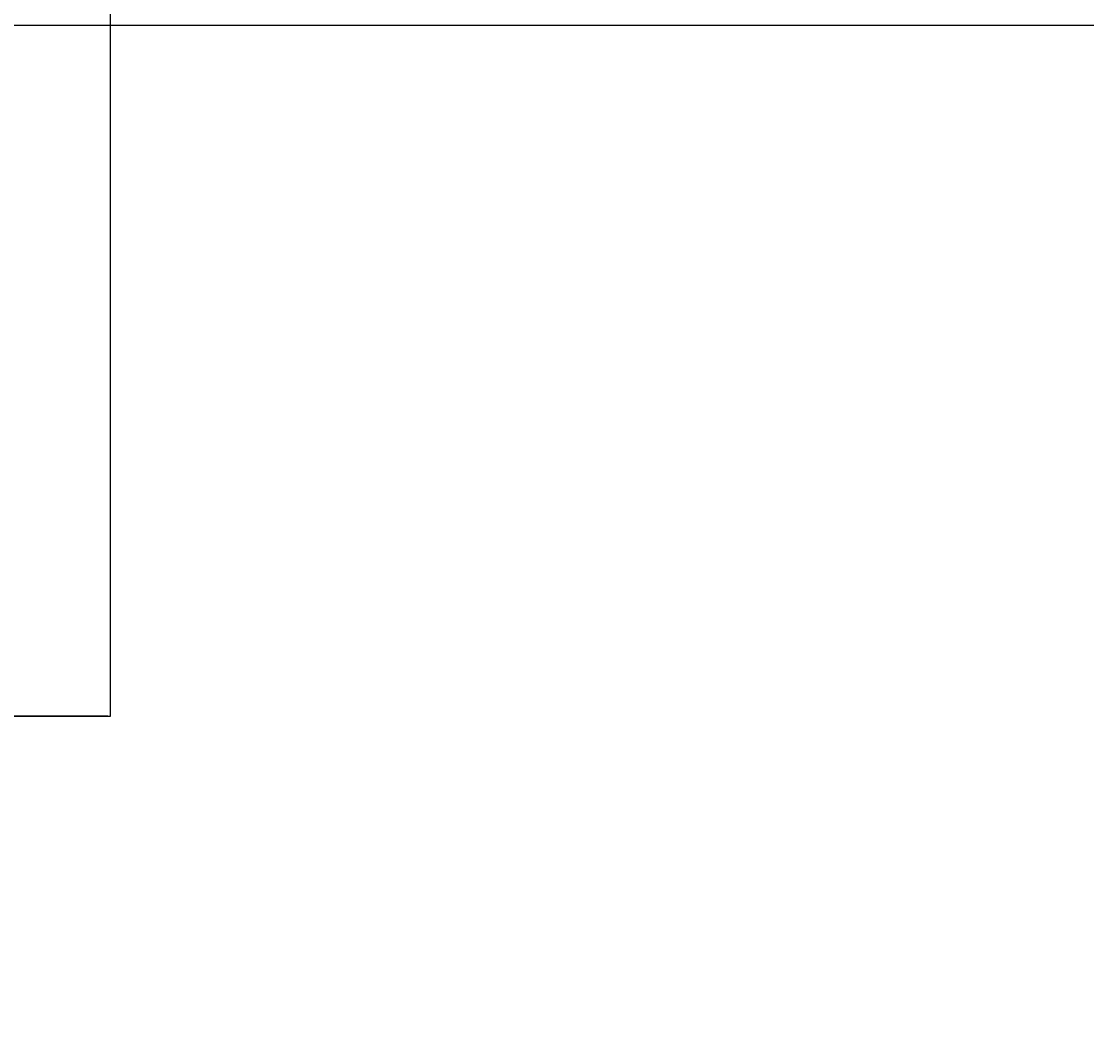
# Model space of a CAD drawing. Units: inches. Extents: x 1998 to 2588, y 1139 to 1977.
# Tile 20 of 134: x 2195 to 2220, y 1605 to 1629. Entities that reach past the tile are written whole.
import ezdxf

# ---------------------------------------------------------------- set-up
doc = ezdxf.new("R2010")
doc.units = ezdxf.units.IN
doc.layers.add('A-ANNO-DIMS', color=2, linetype='Continuous', lineweight=18)
doc.layers.add('A-FLOR-CASE', color=32, linetype='Continuous', lineweight=25)
doc.styles.get("Standard").update_dxf_attribs({"font": 'arial.ttf'})
doc.dimstyles.get("Standard").update_dxf_attribs({"dimtxt": 0.18, "dimasz": 0.18, "dimexe": 0.18, "dimexo": 0.0625, "dimgap": 0.09, "dimtad": 0, "dimtih": 1, "dimtoh": 1, "dimdec": 4, "dimzin": 0, "dimdsep": 46, "dimtxsty": 'Standard', "dimcen": 0.09, "dimadec": 0, "dimazin": 0, "dimtfac": 1, "dimtdec": 4, "dimtofl": 0, "dimtmove": 0, "dimatfit": 3, "dimfxl": 1, "dimtolj": 1, "dimtzin": 0, "dimarcsym": 0})

# ---------------------------------------------------------------- blocks, each defined once
blk = doc.blocks.new('*D30')
at = {"layer": 'A-ANNO-DIMS', "color": 0, "lineweight": -2, "transparency": 16777216}
for p, q in [((2407.91, 1636.732), (1997.843, 1636.732)), ((1998.023, 1636.552), (1998.023, 1615.913)), ((1998.023, 1594.912), (1998.023, 1615.552)), ((2407.91, 1594.732), (1997.843, 1594.732))]:
    blk.add_line(p, q, dxfattribs=at)
at = {"layer": 'A-ANNO-DIMS', "color": 0, "transparency": 16777216}
for points in [[(1997.993, 1636.552), (1998.053, 1636.552), (1998.023, 1636.732)], [(1997.993, 1594.912), (1998.053, 1594.912), (1998.023, 1594.732)]]:
    blk.add_solid(points, dxfattribs=at)
at = {"layer": 'Defpoints', "color": 0, "transparency": 16777216}
for p in [(1998.023, 1636.732), (2407.973, 1636.732), (2407.973, 1594.732)]:
    blk.add_point(p, dxfattribs=at)
at = {"layer": 'A-ANNO-DIMS', "color": 0, "transparency": 16777216, "insert": (1998.023, 1615.732), "char_height": 0.18, "attachment_point": 5}
blk.add_mtext('\\A1;42', dxfattribs=at)
blk = doc.blocks.new('*D37')
at = {"layer": 'A-ANNO-DIMS', "color": 0, "lineweight": -2, "transparency": 16777216}
for p, q in [((2148.455, 1612.795), (2148.455, 1977.362)), ((2197.45, 1612.795), (2197.45, 1977.362)), ((2148.635, 1977.182), (2172.73, 1977.182)), ((2197.27, 1977.182), (2173.175, 1977.182))]:
    blk.add_line(p, q, dxfattribs=at)
at = {"layer": 'A-ANNO-DIMS', "color": 0, "transparency": 16777216}
for points in [[(2148.635, 1977.212), (2148.635, 1977.152), (2148.455, 1977.182)], [(2197.27, 1977.212), (2197.27, 1977.152), (2197.45, 1977.182)]]:
    blk.add_solid(points, dxfattribs=at)
at = {"layer": 'Defpoints', "color": 0, "transparency": 16777216}
for p in [(2197.45, 1977.182), (2148.455, 1612.732), (2197.45, 1612.732)]:
    blk.add_point(p, dxfattribs=at)
at = {"layer": 'A-ANNO-DIMS', "color": 0, "transparency": 16777216, "insert": (2172.952, 1977.182), "char_height": 0.18, "attachment_point": 5}
blk.add_mtext('\\A1;49', dxfattribs=at)
blk = doc.blocks.new('*D38')
at = {"layer": 'A-ANNO-DIMS', "color": 0, "lineweight": -2, "transparency": 16777216}
for p, q in [((2197.387, 1663.247), (1997.843, 1663.247)), ((1998.023, 1663.067), (1998.023, 1638.171)), ((1998.023, 1612.912), (1998.023, 1637.808)), ((2197.387, 1612.732), (1997.843, 1612.732))]:
    blk.add_line(p, q, dxfattribs=at)
at = {"layer": 'A-ANNO-DIMS', "color": 0, "transparency": 16777216}
for points in [[(1997.993, 1663.067), (1998.053, 1663.067), (1998.023, 1663.247)], [(1997.993, 1612.912), (1998.053, 1612.912), (1998.023, 1612.732)]]:
    blk.add_solid(points, dxfattribs=at)
at = {"layer": 'Defpoints', "color": 0, "transparency": 16777216}
for p in [(1998.023, 1663.247), (2197.45, 1663.247), (2197.45, 1612.732)]:
    blk.add_point(p, dxfattribs=at)
at = {"layer": 'A-ANNO-DIMS', "color": 0, "transparency": 16777216, "insert": (1998.023, 1637.99), "char_height": 0.18, "attachment_point": 5}
blk.add_mtext('\\A1;50.51', dxfattribs=at)
blk = doc.blocks.new('*D39')
at = {"layer": 'A-ANNO-DIMS', "color": 0, "lineweight": -2, "transparency": 16777216}
for p, q in [((2115.035, 1628.742), (2588.309, 1628.742)), ((2588.129, 1628.562), (2588.129, 1612.685)), ((2588.129, 1596.444), (2588.129, 1612.321)), ((2115.035, 1596.264), (2588.309, 1596.264))]:
    blk.add_line(p, q, dxfattribs=at)
at = {"layer": 'A-ANNO-DIMS', "color": 0, "transparency": 16777216}
for points in [[(2588.099, 1628.562), (2588.159, 1628.562), (2588.129, 1628.742)], [(2588.099, 1596.444), (2588.159, 1596.444), (2588.129, 1596.264)]]:
    blk.add_solid(points, dxfattribs=at)
at = {"layer": 'Defpoints', "color": 0, "transparency": 16777216}
for p in [(2114.973, 1628.742), (2588.129, 1628.742), (2114.973, 1596.264)]:
    blk.add_point(p, dxfattribs=at)
at = {"layer": 'A-ANNO-DIMS', "color": 0, "transparency": 16777216, "insert": (2588.129, 1612.503), "char_height": 0.18, "attachment_point": 5}
blk.add_mtext('\\A1;32.48', dxfattribs=at)

msp = doc.modelspace()

# ---------------------------------------------------------------- linework, layer by layer
at = {"layer": 'A-FLOR-CASE'}
for p, q in [((2197.4499, 1612.7324), (2197.4499, 1663.2466)), ((2148.4548, 1612.7324), (2197.4499, 1612.7324))]:
    msp.add_line(p, q, dxfattribs=at)

# ---------------------------------------------------------------- dimensions: what is measured, and where the dimension line sits
at = {"layer": 'A-ANNO-DIMS'}
dim = msp.add_linear_dim(base=(2197.4499, 1977.1824), p1=(2148.4548, 1612.7324), p2=(2197.4499, 1612.7324), dimstyle='Standard', override={"dimdec": 0, "dimlfac": 1, "dimrnd": 0, "dimzin": 0, "dimdsep": 46, "dimlunit": 2}, dxfattribs=at)
dim.commit()
dim.dimension.update_dxf_attribs({"geometry": '*D37', "text_midpoint": (2172.9524, 1977.1824)})
for base, p1, p2, override, picture, middle in [((1998.0229, 1663.2466), (2197.4499, 1612.7324), (2197.4499, 1663.2466), {"dimdec": 2, "dimlfac": 1, "dimrnd": 0, "dimzin": 0, "dimdsep": 46, "dimlunit": 2}, '*D38', (1998.0229, 1637.9895)), ((1998.0229, 1636.7324), (2407.9729, 1594.7324), (2407.9729, 1636.7324), {"dimdec": 0, "dimlfac": 1, "dimrnd": 0, "dimzin": 0, "dimdsep": 46, "dimlunit": 2}, '*D30', (1998.0229, 1615.7324)), ((2588.1286, 1628.7416), (2114.9729, 1596.2642), (2114.9729, 1628.7416), {"dimdec": 2, "dimlfac": 1, "dimrnd": 0, "dimzin": 0, "dimdsep": 46, "dimlunit": 2}, '*D39', (2588.1286, 1612.5029))]:
    dim = msp.add_linear_dim(base=base, p1=p1, p2=p2, angle=90, dimstyle='Standard', override=override, dxfattribs=at)
    dim.commit()
    dim.dimension.update_dxf_attribs({"geometry": picture, "text_midpoint": middle})

doc.saveas('drawing.dxf')
